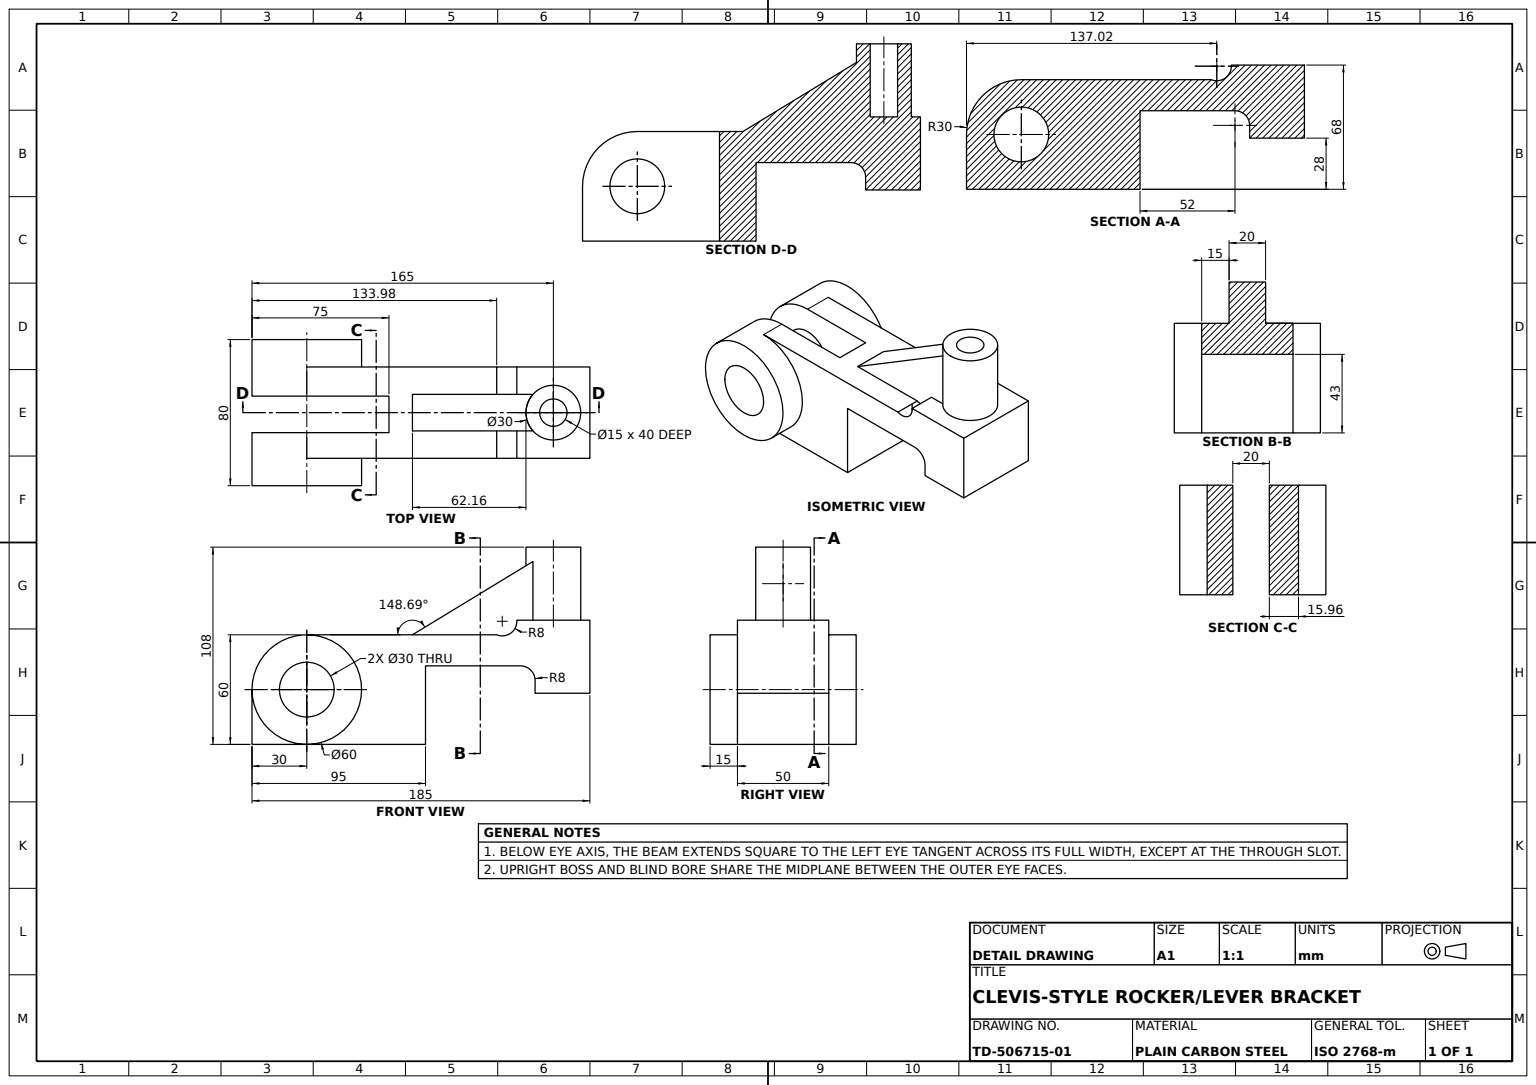
from build123d import *
from build123d.topology import SkipClean

# Parameters (mm, degrees)
ARM_BODY_DEPTH            = 50
FRONT_LUG_SKETCH_R        = 30
FRONT_LUG_SKETCH_R_2      = 15
FRONT_LUG_30_DEPTH        = 15
REAR_START                = 15
REAR_LUG_SKETCH_R         = 30
REAR_LUG_SKETCH_R_2       = 15
REAR_LUG_30_DEPTH         = 15
TOP_SLOT_SKETCH_W         = 75
TOP_SLOT_SKETCH_H         = 20
TOP_SLOT_CUT_DEPTH        = 179.465683
LUG_RELIEF_CUT_DEPTH      = 173.771525
PIN_POST_SKETCH_R         = 15
PIN_POST_SKETCH_R_2       = 7.5
PIN_POST_15_DEPTH         = 40
SUPPORT_RIB_REACH         = 180.955
SUPPORT_RIB_SKETCH_WALL_W = 432.658256
SUPPORT_RIB_SKETCH_WALL_H = 20
EYE_BORE_SKETCH_R         = 15
EYE_BORE_DEPTH            = 187.145105


with BuildPart() as part:
    # Arm Profile Sketch → Arm Body (new body)
    with BuildSketch(Plane.XY):
        with BuildLine():
            Line((0, 0), (30, 0))
            Line((30, 0), (30, 40))
            Line((30, 40), (-10, 40))
            ThreePointArc((-10, 40), (-13.278154, 32.923449), (-21.022255, 32))
            Line((-21.022255, 32), (-155, 32))
            Line((-155, 32), (-155, -28))
            Line((-155, -28), (-60, -28))
            Line((-60, -28), (-60, 15))
            Line((-60, 15), (-8, 15))
            ThreePointArc((-8, 15), (-2.343146, 12.656854), (0, 7))
            Line((0, 7), (0, 0))
        make_face()
    extrude(amount=ARM_BODY_DEPTH)

    # Front Lug Sketch → Front Lug Ø30 (add)
    with BuildSketch(Plane.XY.offset(50)):
        with Locations(Location((-125, 2, 0), (0, 0, 180))):
            Circle(FRONT_LUG_SKETCH_R)
        with Locations((-125, 2)):
            Circle(FRONT_LUG_SKETCH_R_2, mode=Mode.SUBTRACT)
    extrude(amount=FRONT_LUG_30_DEPTH)

    # Rear Lug Sketch → Rear Lug Ø30 (add)
    with BuildSketch(Plane(origin=(0, 0, 0), x_dir=(-1, 0, 0), z_dir=(0, 0, -1)).offset(REAR_START)):
        with Locations((125, 2)):
            Circle(REAR_LUG_SKETCH_R)
        with Locations(Location((125, 2, 0), (0, 0, 180))):
            Circle(REAR_LUG_SKETCH_R_2, mode=Mode.SUBTRACT)
    extrude(amount=-REAR_LUG_30_DEPTH)

    # Top Slot Sketch → Top Slot Cut (cut, through all)
    with BuildSketch(Plane(origin=(0, 32, 0), x_dir=(1, 0, 0), z_dir=(0, 1, 0))):
        with Locations((-117.5, -25.955312)):
            Rectangle(TOP_SLOT_SKETCH_W, TOP_SLOT_SKETCH_H)
    extrude(amount=-TOP_SLOT_CUT_DEPTH, mode=Mode.SUBTRACT)

    # Lug Relief Sketch → Lug Relief Cut (cut, through all)
    with SkipClean():  # the faces are left unmerged after this step: merging them gives an invalid solid
        with BuildSketch(Plane.XY.offset(50)):
            with BuildLine():
                Line((-155, 32), (-125, 32))
                ThreePointArc((-125, 32), (-146.213203, 23.213203), (-155, 2))
                Line((-155, 2), (-155, 32))
            make_face()
        extrude(amount=-LUG_RELIEF_CUT_DEPTH, mode=Mode.SUBTRACT)

    # Pin Post Sketch → Pin Post Ø15 (add)
    with SkipClean():  # the faces are left unmerged after this step: merging them gives an invalid solid
        with BuildSketch(Plane(origin=(0, 40, 0), x_dir=(1, 0, 0), z_dir=(0, 1, 0))):
            with Locations(Location((10, -25, 0), (0, 0, 90))):
                Circle(PIN_POST_SKETCH_R)
            with Locations(Location((10, -25, 0), (0, 0, 270))):
                Circle(PIN_POST_SKETCH_R_2, mode=Mode.SUBTRACT)
        extrude(amount=PIN_POST_15_DEPTH)

    # Support Rib Sketch wall → Support Rib (add, up to next)
    with BuildSketch(Plane(origin=(-36.077613, 50.900721, 25), x_dir=(-0.854394921364, -0.519624208778, 0), z_dir=(0.519624208778, -0.854394921364, 0)), mode=Mode.PRIVATE) as support_rib_sk1:
        Rectangle(SUPPORT_RIB_SKETCH_WALL_W, SUPPORT_RIB_SKETCH_WALL_H)
    support_rib_tool1 = extrude(support_rib_sk1.sketch, amount=SUPPORT_RIB_REACH, mode=Mode.PRIVATE) - part.part
    add(support_rib_tool1.solids().sort_by_distance((-36.077613, 50.900721, 25))[0])

    # Eye Bore Sketch → Eye Bore (cut, through all)
    with SkipClean():  # the faces are left unmerged after this step: merging them gives an invalid solid
        with BuildSketch(Plane.XY.offset(50)):
            with Locations((-125, 2)):
                Circle(EYE_BORE_SKETCH_R)
        extrude(amount=-EYE_BORE_DEPTH, mode=Mode.SUBTRACT)


solid = part.part
